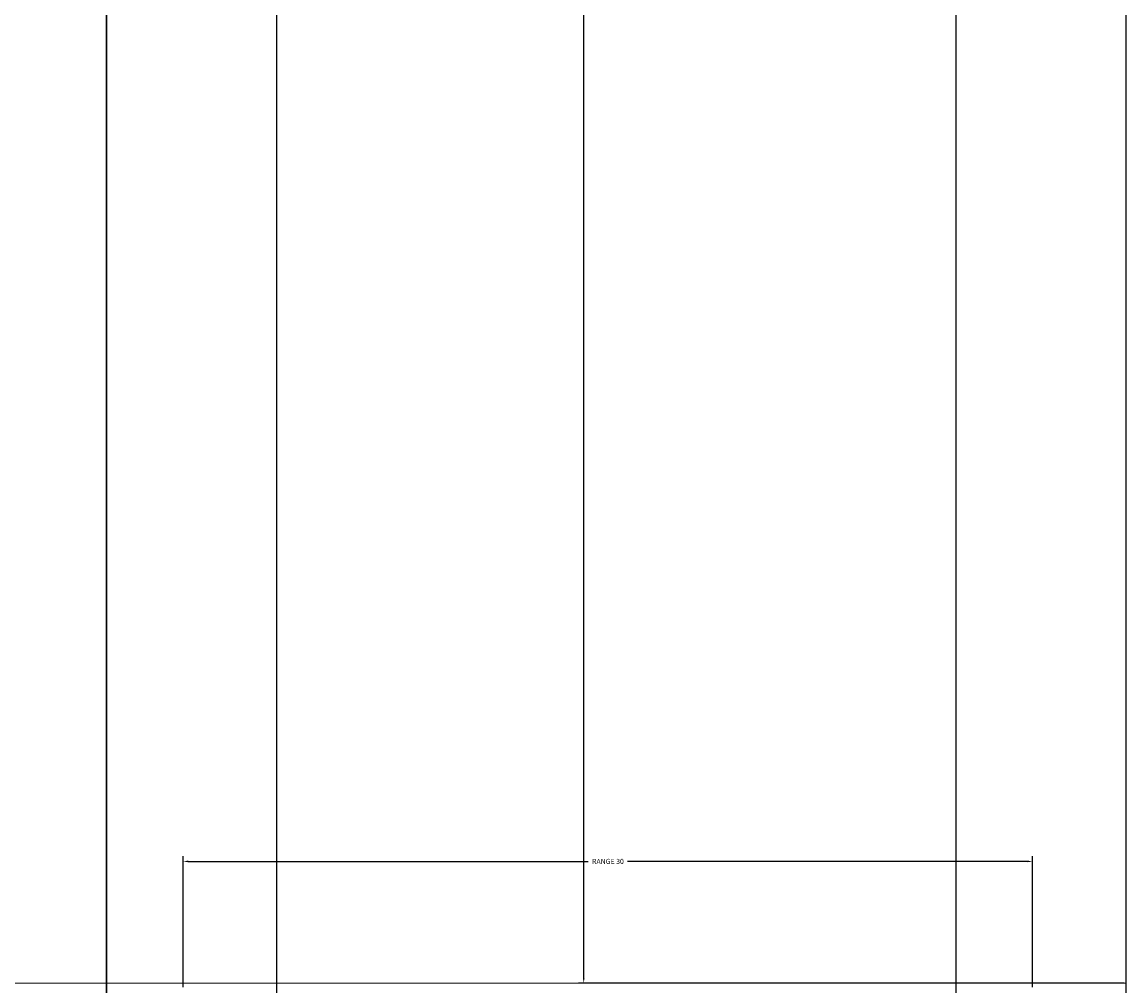
# Model space of a CAD drawing. Units: inches. Extents: x 2307 to 2544, y 2171 to 2540.
# Tile 32 of 52: x 2453 to 2492, y 2343 to 2377. Entities that reach past the tile are written whole.
import ezdxf

# ---------------------------------------------------------------- set-up
doc = ezdxf.new("R2010")
doc.units = ezdxf.units.IN
doc.layers.add('A-ANNO-DIMS', color=2, linetype='Continuous', lineweight=18)
doc.layers.add('A-FLOR-CASE', color=9, linetype='Continuous', lineweight=18)
doc.styles.get("Standard").update_dxf_attribs({"font": 'arial.ttf'})
doc.dimstyles.get("Standard").update_dxf_attribs({"dimtxt": 0.18, "dimasz": 0.18, "dimexe": 0.18, "dimexo": 0.0625, "dimgap": 0.09, "dimtad": 0, "dimtih": 1, "dimtoh": 1, "dimdec": 4, "dimzin": 0, "dimdsep": 46, "dimtxsty": 'Standard', "dimcen": 0.09, "dimadec": 0, "dimazin": 0, "dimtfac": 1, "dimtdec": 4, "dimtofl": 0, "dimtmove": 0, "dimatfit": 3, "dimfxl": 1, "dimtolj": 1, "dimtzin": 0, "dimarcsym": 0})

# ---------------------------------------------------------------- blocks, each defined once
blk = doc.blocks.new('*D30')
at = {"layer": 'A-ANNO-DIMS', "color": 0, "lineweight": -2, "transparency": 16777216}
for p, q in [((2458.401, 2343.369), (2458.401, 2347.987)), ((2488.401, 2343.369), (2488.401, 2347.987)), ((2458.581, 2347.807), (2472.705, 2347.807)), ((2488.221, 2347.807), (2474.097, 2347.807))]:
    blk.add_line(p, q, dxfattribs=at)
at = {"layer": 'A-ANNO-DIMS', "color": 0, "transparency": 16777216}
for points in [[(2458.581, 2347.837), (2458.581, 2347.777), (2458.401, 2347.807)], [(2488.221, 2347.837), (2488.221, 2347.777), (2488.401, 2347.807)]]:
    blk.add_solid(points, dxfattribs=at)
at = {"layer": 'Defpoints', "color": 0, "transparency": 16777216}
for p in [(2458.401, 2347.807), (2458.401, 2343.307), (2488.401, 2343.307)]:
    blk.add_point(p, dxfattribs=at)
at = {"layer": 'A-ANNO-DIMS', "color": 0, "transparency": 16777216, "insert": (2473.401, 2347.807), "char_height": 0.18, "attachment_point": 5}
blk.add_mtext('\\A1;RANGE 30', dxfattribs=at)
blk = doc.blocks.new('*D49')
at = {"layer": 'A-ANNO-DIMS', "color": 0, "lineweight": -2, "transparency": 16777216}
for p, q in [((2491.633, 2435.51), (2472.366, 2435.51)), ((2472.546, 2435.33), (2472.546, 2389.691)), ((2472.546, 2343.69), (2472.546, 2389.328)), ((2491.633, 2343.51), (2472.366, 2343.51))]:
    blk.add_line(p, q, dxfattribs=at)
at = {"layer": 'A-ANNO-DIMS', "color": 0, "transparency": 16777216}
for points in [[(2472.516, 2435.33), (2472.576, 2435.33), (2472.546, 2435.51)], [(2472.516, 2343.69), (2472.576, 2343.69), (2472.546, 2343.51)]]:
    blk.add_solid(points, dxfattribs=at)
at = {"layer": 'Defpoints', "color": 0, "transparency": 16777216}
for p in [(2472.546, 2435.51), (2491.696, 2435.51), (2491.696, 2343.51)]:
    blk.add_point(p, dxfattribs=at)
at = {"layer": 'A-ANNO-DIMS', "color": 0, "transparency": 16777216, "insert": (2472.546, 2389.51), "char_height": 0.18, "attachment_point": 5}
blk.add_mtext('\\A1;92', dxfattribs=at)
blk = doc.blocks.new('*D53')
at = {"layer": 'A-ANNO-DIMS', "color": 0, "lineweight": -2, "transparency": 16777216}
for p, q in [((2455.696, 2439.447), (2455.696, 2171.18)), ((2461.696, 2439.447), (2461.696, 2171.18)), ((2455.876, 2171.36), (2458.546, 2171.36)), ((2461.516, 2171.36), (2458.845, 2171.36))]:
    blk.add_line(p, q, dxfattribs=at)
at = {"layer": 'A-ANNO-DIMS', "color": 0, "transparency": 16777216}
for points in [[(2455.876, 2171.39), (2455.876, 2171.33), (2455.696, 2171.36)], [(2461.516, 2171.39), (2461.516, 2171.33), (2461.696, 2171.36)]]:
    blk.add_solid(points, dxfattribs=at)
at = {"layer": 'Defpoints', "color": 0, "transparency": 16777216}
for p in [(2455.696, 2439.51), (2461.696, 2439.51), (2461.696, 2171.36)]:
    blk.add_point(p, dxfattribs=at)
at = {"layer": 'A-ANNO-DIMS', "color": 0, "transparency": 16777216, "insert": (2458.696, 2171.36), "char_height": 0.18, "attachment_point": 5}
blk.add_mtext('\\A1;6', dxfattribs=at)
blk = doc.blocks.new('*D54')
at = {"layer": 'A-ANNO-DIMS', "color": 0, "lineweight": -2, "transparency": 16777216}
for p, q in [((2461.696, 2435.447), (2461.696, 2171.18)), ((2491.696, 2435.447), (2491.696, 2171.18)), ((2461.876, 2171.36), (2476.477, 2171.36)), ((2491.516, 2171.36), (2476.914, 2171.36))]:
    blk.add_line(p, q, dxfattribs=at)
at = {"layer": 'A-ANNO-DIMS', "color": 0, "transparency": 16777216}
for points in [[(2461.876, 2171.39), (2461.876, 2171.33), (2461.696, 2171.36)], [(2491.516, 2171.39), (2491.516, 2171.33), (2491.696, 2171.36)]]:
    blk.add_solid(points, dxfattribs=at)
at = {"layer": 'Defpoints', "color": 0, "transparency": 16777216}
for p in [(2461.696, 2435.51), (2491.696, 2435.51), (2491.696, 2171.36)]:
    blk.add_point(p, dxfattribs=at)
at = {"layer": 'A-ANNO-DIMS', "color": 0, "transparency": 16777216, "insert": (2476.696, 2171.36), "char_height": 0.18, "attachment_point": 5}
blk.add_mtext('\\A1;30', dxfattribs=at)
blk = doc.blocks.new('*D59')
at = {"layer": 'A-ANNO-DIMS', "color": 0, "lineweight": -2, "transparency": 16777216}
for p, q in [((2455.696, 2315.572), (2455.696, 2540.345)), ((2455.876, 2540.165), (2470.477, 2540.165)), ((2485.516, 2540.165), (2470.914, 2540.165)), ((2485.696, 2315.572), (2485.696, 2540.345))]:
    blk.add_line(p, q, dxfattribs=at)
at = {"layer": 'A-ANNO-DIMS', "color": 0, "transparency": 16777216}
for points in [[(2455.876, 2540.195), (2455.876, 2540.135), (2455.696, 2540.165)], [(2485.516, 2540.195), (2485.516, 2540.135), (2485.696, 2540.165)]]:
    blk.add_solid(points, dxfattribs=at)
at = {"layer": 'Defpoints', "color": 0, "transparency": 16777216}
for p in [(2455.696, 2540.165), (2455.696, 2315.51), (2485.696, 2315.51)]:
    blk.add_point(p, dxfattribs=at)
at = {"layer": 'A-ANNO-DIMS', "color": 0, "transparency": 16777216, "insert": (2470.696, 2540.165), "char_height": 0.18, "attachment_point": 5}
blk.add_mtext('\\A1;30', dxfattribs=at)

msp = doc.modelspace()

# ---------------------------------------------------------------- linework, layer by layer
at = {"layer": 'A-FLOR-CASE'}
for p, q in [((2491.6958, 2435.5096), (2491.6958, 2343.5096)), ((2491.6958, 2343.5096), (2451.6958, 2343.5096))]:
    msp.add_line(p, q, dxfattribs=at)

# ---------------------------------------------------------------- dimensions: what is measured, and where the dimension line sits
at = {"layer": 'A-ANNO-DIMS'}
for base, p1, p2, picture, middle in [((2455.6958, 2540.1649), (2485.6958, 2315.5096), (2455.6958, 2315.5096), '*D59', (2470.6958, 2540.1649)), ((2461.6958, 2171.3596), (2455.6958, 2439.5096), (2461.6958, 2439.5096), '*D53', (2458.6958, 2171.3596)), ((2491.6958, 2171.3596), (2461.6958, 2435.5096), (2491.6958, 2435.5096), '*D54', (2476.6958, 2171.3596))]:
    dim = msp.add_linear_dim(base=base, p1=p1, p2=p2, dimstyle='Standard', override={"dimdec": 0, "dimlfac": 1, "dimrnd": 0, "dimzin": 0, "dimdsep": 46, "dimlunit": 2}, dxfattribs=at)
    dim.commit()
    dim.dimension.update_dxf_attribs({"geometry": picture, "text_midpoint": middle})
dim = msp.add_linear_dim(base=(2472.5458, 2435.5096), p1=(2491.6958, 2343.5096), p2=(2491.6958, 2435.5096), angle=90, dimstyle='Standard', override={"dimdec": 0, "dimlfac": 1, "dimrnd": 0, "dimzin": 0, "dimdsep": 46, "dimlunit": 2}, dxfattribs=at)
dim.commit()
dim.dimension.update_dxf_attribs({"geometry": '*D49', "text_midpoint": (2472.5458, 2389.5096)})
dim = msp.add_linear_dim(base=(2458.4011, 2347.8068), p1=(2488.4011, 2343.3068), p2=(2458.4011, 2343.3068), angle=180, text='RANGE <>', dimstyle='Standard', override={"dimdec": 0, "dimlfac": 1, "dimrnd": 0, "dimzin": 0, "dimdsep": 46, "dimlunit": 2}, dxfattribs=at)
dim.commit()
dim.dimension.update_dxf_attribs({"geometry": '*D30', "text_midpoint": (2473.4011, 2347.8068)})

doc.saveas('drawing.dxf')
